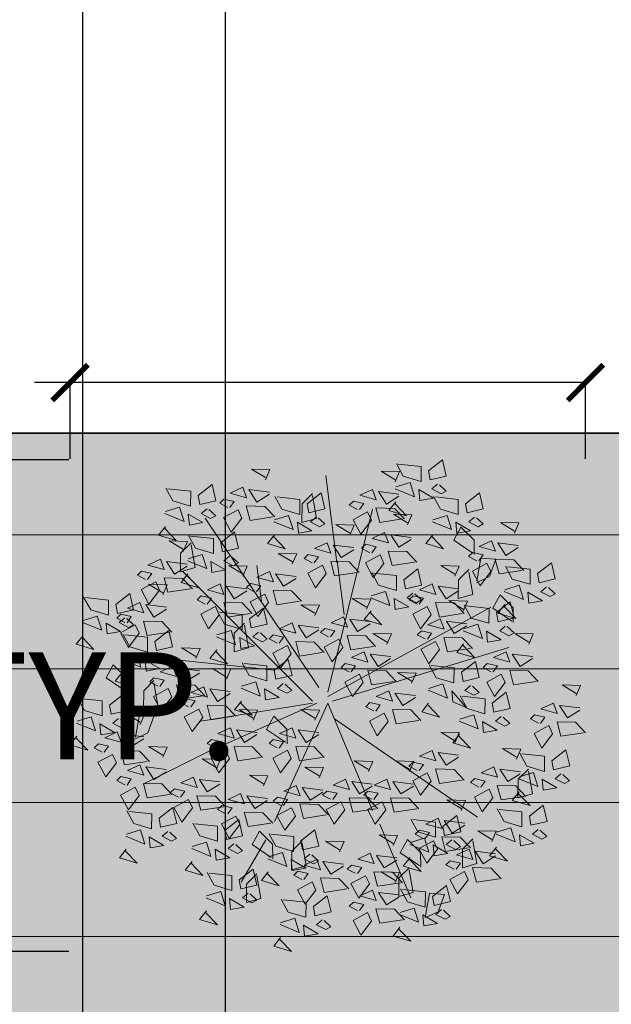
# Model space of a CAD drawing. Units: inches. Extents: x 1704 to 6393, y -157 to 1172.
# Tile 102 of 122: x 2594 to 2627, y 1001 to 1056. Entities that reach past the tile are written whole.
import ezdxf

# ---------------------------------------------------------------- set-up
doc = ezdxf.new("R2010")
doc.units = ezdxf.units.IN
doc.header["$MEASUREMENT"] = 0
for name, color, linetype, lineweight in [('A-ANNO-DIMS', 7, 'Continuous', 13), ('C-PROP', 7, 'Continuous', 35), ('L-DECK-PLNK-PATT', 250, 'Continuous', 13), ('L-shrub', 74, 'Continuous', 18)]:
    doc.layers.add(name, color=color, linetype=linetype, lineweight=lineweight)
doc.layers.add('L-DECK-PATT', color=35, linetype='Continuous', lineweight=13, true_color=0xa6725b)
doc.styles.get("Standard").update_dxf_attribs({"font": 'arial.ttf'})
doc.dimstyles.get("Standard").update_dxf_attribs({"dimtxt": 6, "dimasz": 2, "dimexe": 0.18, "dimexo": 0.0625, "dimgap": 0.09, "dimtad": 0, "dimtih": 1, "dimtoh": 1, "dimdec": 1, "dimzin": 0, "dimdsep": 46, "dimlunit": 3, "dimtxsty": 'Standard', "dimblk": 'ARCHTICK', "dimcen": 0.09, "dimadec": 0, "dimazin": 0, "dimtfac": 1, "dimtdec": 1, "dimtofl": 0, "dimtmove": 0, "dimatfit": 3, "dimfxl": 1, "dimtolj": 1, "dimtzin": 0, "dimarcsym": 0})

# ---------------------------------------------------------------- blocks, each defined once
blk = doc.blocks.new('flower shrub 3')
at = {"layer": 'L-shrub'}
for p, q in [((-123.5, 236), (-109, 242.8)), ((-109.8, 240.6), (-114, 215.7)), ((-130.4, 216.9), (-123.5, 236)), ((-114, 215.7), (-130.4, 216.9)), ((-96, 214.8), (-80.2, 219.2)), ((-80.2, 219.2), (-80.3, 198.9)), ((71.1, 221.6), (86.9, 226)), ((75.6, 196.7), (71.1, 221.6)), ((86.9, 226), (86.9, 205.7)), ((-91.6, 189.9), (-96, 214.8)), ((86.9, 205.7), (75.5, 194.4)), ((-80.3, 198.9), (-91.6, 187.7)), ((-166.1, 183.2), (-150.2, 187.7)), ((-150.2, 187.7), (-150.3, 167.3)), ((-104.3, 171), (-104.5, 187)), ((-102.9, 185.4), (-82, 171.2)), ((21.4, 185.5), (37.3, 189.9)), ((25.9, 160.6), (21.4, 185.5)), ((37.3, 189.9), (37.2, 169.6)), ((-161.6, 158.3), (-166.1, 183.2)), ((58.3, 162), (58.1, 177.9)), ((59.8, 176.3), (80.7, 162.2)), ((-150.3, 167.3), (-161.6, 156.1)), ((-89.8, 156.8), (-104.3, 171)), ((-82, 171.2), (-89.8, 156.8)), ((37.2, 169.6), (25.8, 158.3)), ((80.7, 162.2), (72.8, 147.7)), ((72.8, 147.7), (58.3, 162)), ((-227, 106.5), (-211.2, 110.9)), ((-211.2, 110.9), (-211.3, 90.6)), ((-222.6, 81.6), (-227, 106.5)), ((-211.3, 90.6), (-222.6, 79.4)), ((42.5, 35.6), (42.3, 51.6)), ((43.9, 50), (64.8, 35.8)), ((195.1, 39.7), (209.5, 46.5)), ((208.7, 44.3), (204.5, 19.5)), ((57, 21.4), (42.5, 35.6)), ((64.8, 35.8), (57, 21.4)), ((188.1, 20.6), (195.1, 39.7)), ((184.1, 9.5), (199.9, 13.9)), ((204.5, 19.5), (188.1, 20.6)), ((199.9, 13.9), (199.8, -6.4)), ((188.5, -15.4), (184.1, 9.5)), ((199.8, -6.4), (188.5, -17.7)), ((218.7, -20.8), (218.5, -4.8)), ((220.1, -6.4), (241, -20.6)), ((233.2, -35), (218.7, -20.8)), ((241, -20.6), (233.2, -35)), ((84.7, -53.7), (100.5, -49.2)), ((89.1, -78.6), (84.7, -53.7)), ((100.5, -49.2), (100.4, -69.6)), ((100.4, -69.6), (89.1, -80.8)), ((-206, -97.5), (-206.1, -81.5)), ((-204.5, -83.1), (-183.6, -97.3)), ((-191.5, -111.7), (-206, -97.5)), ((-183.6, -97.3), (-191.5, -111.7)), ((-161.5, -112.4), (-145.7, -107.9)), ((-145.7, -107.9), (-145.8, -128.2)), ((-157.1, -137.2), (-161.5, -112.4)), ((-179.9, -131.8), (-165.5, -125)), ((-166.2, -127.1), (-170.5, -152)), ((-145.8, -128.2), (-157.1, -139.5)), ((-186.9, -150.9), (-179.9, -131.8)), ((143.4, -141.7), (159.2, -137.2)), ((159.2, -137.2), (159.2, -157.6)), ((-170.5, -152), (-186.9, -150.9)), ((147.8, -166.6), (143.4, -141.7)), ((-163.1, -171.9), (-163.2, -156)), ((-161.6, -157.6), (-140.7, -171.7)), ((159.2, -157.6), (147.8, -168.8)), ((-148.6, -186.2), (-163.1, -171.9)), ((-140.7, -171.7), (-148.6, -186.2)), ((10.1, -195.8), (26, -191.4)), ((26, -191.4), (25.9, -211.7)), ((14.6, -220.7), (10.1, -195.8)), ((25.9, -211.7), (14.5, -223))]:
    blk.add_line(p, q, dxfattribs=at)
for points in [[(49.5, 264.4), (57, 273.9), (37.6, 279.7), (50.2, 266.6)], [(-81.5, 253.1), (-74, 262.7), (-93.5, 268.4), (-80.9, 255.3)], [(-50.4, 246.2), (-38.7, 261.6), (-30.1, 245.6), (-46.1, 237), (-50.4, 246.2)], [(24.3, 250.7), (23.1, 262.8), (8.2, 260.2), (24.3, 250.7)], [(-106.8, 239.4), (-107.9, 251.5), (-122.8, 248.9), (-106.8, 239.4)], [(-84.3, 244.8), (-59.4, 248.7), (-55.3, 232.7), (-75.6, 233.3), (-86.6, 244.9)], [(3.7, 245), (10, 250.2), (-0.2, 255.6), (-5.8, 252.5), (1.6, 245.7)], [(49.4, 248), (33.8, 243.2), (29, 258.7), (50, 250.1)], [(130.8, 235.1), (138.4, 244.6), (118.9, 250.4), (131.5, 237.2)], [(-127.3, 233.7), (-121, 238.9), (-131.2, 244.3), (-136.8, 241.3), (-129.5, 234.4)], [(-81.7, 236.7), (-97.2, 231.9), (-102, 247.4), (-81, 238.9)], [(13.5, 230.4), (-1.8, 218.4), (-6, 236.1), (11.8, 240.3), (13.5, 230.4)], [(46.7, 222.9), (21.5, 225.6), (21.7, 242.1), (41.2, 236.3), (48.8, 222.3)], [(-117.5, 219.1), (-132.8, 207.1), (-137, 224.8), (-119.3, 229), (-117.5, 219.1)], [(-84.4, 211.6), (-109.5, 214.3), (-109.3, 230.8), (-89.8, 225), (-82.2, 211)], [(-80.5, 219.9), (-66.7, 228.5), (-58, 214.8), (-80.5, 217.6)], [(-37.1, 234.5), (-41.8, 227.9), (-30.6, 225.3), (-26, 229.7), (-34.9, 234.5)], [(10.6, 212.3), (22.3, 227.8), (30.9, 211.8), (14.9, 203.2), (10.6, 212.3)], [(105.6, 221.4), (104.4, 233.5), (89.5, 230.8), (105.6, 221.4)], [(130.7, 218.7), (115.1, 213.8), (110.3, 229.4), (131.3, 220.8)], [(-156.6, 201), (-144.8, 216.5), (-136.2, 200.5), (-152.3, 191.9), (-156.6, 201)], [(-59.4, 140), (-93.7, 220.8)], [(-55.5, 223.7), (-51.3, 212.3), (-37.6, 218.7), (-55.5, 223.7)], [(-48.1, 205.5), (-36.4, 221), (-27.8, 205), (-43.9, 196.4), (-48.1, 205.5)], [(85, 215.7), (91.3, 220.9), (81.1, 226.3), (75.5, 223.2), (82.9, 216.3)], [(-82.1, 204.2), (-57.1, 208), (-53, 192.1), (-73.3, 192.7), (-84.3, 204.3)], [(-23.3, 211), (1.6, 214.8), (5.7, 198.9), (-14.6, 199.5), (-25.6, 211)], [(63.1, 192.2), (70.6, 201.7), (51.1, 207.5), (63.7, 194.4)], [(94.8, 201), (79.5, 189.1), (75.4, 206.8), (93.1, 211), (94.8, 201)], [(128, 193.6), (102.9, 196.3), (103, 212.7), (122.5, 207), (130.1, 192.9)], [(-190.5, 199.7), (-165.5, 203.5), (-161.4, 187.6), (-181.8, 188.2), (-192.7, 199.8)], [(-76.4, 204), (-81.2, 192.8), (-60.9, 192.3), (-76.4, 201.7)], [(-19.5, 186), (-5.7, 194.7), (3, 180.9), (-19.5, 183.8)], [(23.9, 200.7), (19.2, 194), (30.4, 191.5), (35, 195.9), (26.1, 200.6)], [(65.7, 157.2), (92.6, 203.7)], [(146.6, 180.9), (154.2, 190.5), (134.7, 196.2), (147.3, 183.1)], [(-143.3, 189.4), (-148, 182.7), (-136.8, 180.2), (-132.1, 184.6), (-141, 189.3)], [(-92.8, 176.4), (-85.3, 186), (-104.8, 191.7), (-92.2, 178.6)], [(-78.2, 179.3), (-64.4, 187.9), (-55.7, 174.2), (-78.3, 177)], [(-34.9, 193.9), (-39.6, 187.3), (-28.3, 184.7), (-23.7, 189.1), (-32.6, 193.8)], [(5.5, 189.9), (9.7, 178.5), (23.4, 184.9), (5.5, 189.9)], [(37.8, 178.5), (36.7, 190.6), (21.8, 188), (37.8, 178.5)], [(62.9, 175.8), (47.4, 171), (42.5, 186.5), (63.6, 177.9)], [(-187.7, 165.1), (-180.1, 174.7), (-199.6, 180.4), (-187, 167.3)], [(-186.6, 174.8), (-172.8, 183.4), (-164.2, 169.6), (-186.7, 172.5)], [(-161.7, 178.6), (-157.5, 167.2), (-143.7, 173.6), (-161.7, 178.6)], [(-118.1, 162.7), (-119.2, 174.8), (-134.1, 172.2), (-118.1, 162.7)], [(-122.7, 167.2), (-111, 182.7), (-102.3, 166.6), (-118.4, 158), (-122.7, 167.2)], [(-53.2, 183.1), (-49, 171.7), (-35.3, 178.1), (-53.2, 183.1)], [(17.3, 172.8), (23.5, 178), (13.3, 183.4), (7.7, 180.4), (15.1, 173.5)], [(121.4, 167.2), (120.3, 179.3), (105.3, 176.7), (121.4, 167.2)], [(146.5, 164.5), (130.9, 159.7), (126.1, 175.2), (147.1, 166.7)], [(218.9, 167.4), (226.5, 176.9), (207, 182.7), (219.6, 169.6)], [(-212.9, 151.4), (-214.1, 163.5), (-229, 160.9), (-212.9, 151.4)], [(-156.6, 165.8), (-131.6, 169.7), (-127.5, 153.8), (-147.9, 154.3), (-158.9, 165.9)], [(-138.6, 157), (-132.3, 162.2), (-142.5, 167.6), (-148.1, 164.6), (-140.8, 157.7)], [(-92.9, 160), (-108.5, 155.2), (-113.3, 170.7), (-92.3, 162.2)], [(-74.1, 163.4), (-78.9, 152.2), (-58.6, 151.7), (-74.2, 161.1)], [(-15.4, 170.1), (-20.2, 159), (0.1, 158.4), (-15.4, 167.9)], [(27.1, 158.2), (11.8, 146.2), (7.6, 163.9), (25.3, 168.1), (27.1, 158.2)], [(60.2, 150.7), (35.1, 153.4), (35.3, 169.9), (54.7, 164.1), (62.4, 150.1)], [(100.9, 161.5), (107.1, 166.7), (96.9, 172.1), (91.3, 169.1), (98.7, 162.2)], [(193.7, 153.7), (192.5, 165.8), (177.6, 163.1), (193.7, 153.7)], [(-233.5, 145.7), (-227.2, 151), (-237.4, 156.3), (-243, 153.3), (-235.6, 146.4)], [(-187.8, 148.7), (-203.4, 143.9), (-208.2, 159.4), (-187.2, 150.9)], [(-182.5, 158.9), (-187.4, 147.7), (-167, 147.1), (-182.6, 156.6)], [(-128.8, 142.4), (-144.1, 130.4), (-148.3, 148.1), (-130.6, 152.3), (-128.8, 142.4)], [(-95.7, 134.9), (-120.8, 137.6), (-120.6, 154.1), (-101.1, 148.3), (-93.5, 134.3)], [(-109.4, 155.5), (-114.1, 148.9), (-102.9, 146.3), (-98.3, 150.7), (-107.2, 155.5)], [(110.7, 146.9), (95.3, 134.9), (91.2, 152.6), (108.9, 156.8), (110.7, 146.9)], [(94.2, 140.1), (105.9, 155.6), (114.5, 139.6), (98.5, 131), (94.2, 140.1)], [(143.8, 139.4), (118.7, 142.1), (118.8, 158.6), (138.3, 152.8), (146, 138.8)], [(173.1, 148), (179.4, 153.2), (169.2, 158.6), (163.6, 155.5), (171, 148.6)], [(218.8, 151), (203.2, 146.2), (198.4, 161.7), (219.4, 153.1)], [(-223.7, 131.1), (-239, 119.1), (-243.2, 136.9), (-225.4, 141), (-223.7, 131.1)], [(-190.5, 123.6), (-215.6, 126.4), (-215.5, 142.8), (-196, 137), (-188.4, 123)], [(-152.8, 140.9), (-139, 149.6), (-130.3, 135.8), (-152.8, 138.7)], [(-127.8, 144.8), (-123.6, 133.4), (-109.9, 139.8), (-127.8, 144.8)], [(33.2, 131.1), (44.9, 146.6), (53.5, 130.5), (37.5, 121.9), (33.2, 131.1)], [(60.3, 138.8), (85.2, 142.6), (89.3, 126.7), (69, 127.3), (58, 138.8)], [(182.9, 133.3), (167.6, 121.4), (163.4, 139.1), (181.2, 143.3), (182.9, 133.3)], [(216.1, 125.9), (191, 128.6), (191.1, 145), (210.6, 139.3), (218.2, 125.2)], [(-9.9, 24.3), (-166.8, 132)], [(-66.2, 124.3), (-54.5, 139.8), (-45.9, 123.8), (-61.9, 115.2), (-66.2, 124.3)], [(-21, 124.3), (-9.3, 139.8), (-0.7, 123.8), (-16.7, 115.2), (-21, 124.3)], [(-0.7, 129.8), (24.2, 133.6), (28.3, 117.7), (8, 118.2), (-3, 129.8)], [(-2.5, 7.1), (56.3, 136.9)], [(146.1, 122.1), (157.9, 137.6), (166.5, 121.5), (150.4, 112.9), (146.1, 122.1)], [(-212.5, 104.2), (-205, 113.8), (-224.5, 119.5), (-211.9, 106.4)], [(-183.7, 110.8), (-171.9, 126.3), (-163.3, 110.2), (-179.4, 101.6), (-183.7, 110.8)], [(-148.7, 125), (-153.5, 113.9), (-133.2, 113.3), (-148.7, 122.8)], [(-100.1, 123), (-75.2, 126.8), (-71.1, 110.9), (-91.4, 111.5), (-102.4, 123)], [(-54.9, 123), (-30, 126.8), (-25.9, 110.9), (-46.2, 111.5), (-57.2, 123)], [(-2.5, 7.1), (-51.6, 124.7)], [(46.4, 119.4), (41.7, 112.8), (53, 110.2), (57.6, 114.6), (48.7, 119.4)], [(64.1, 113.8), (77.9, 122.5), (86.6, 108.7), (64, 111.6)], [(107.4, 128.5), (102.7, 121.8), (114, 119.3), (118.6, 123.7), (109.7, 128.4)], [(112.2, 120.7), (137.2, 124.6), (141.3, 108.7), (120.9, 109.2), (110, 120.8)], [(204.9, 108.5), (216.6, 124), (225.2, 108), (209.2, 99.4), (204.9, 108.5)], [(-217.6, 109.4), (-192.6, 113.3), (-188.5, 97.4), (-208.9, 97.9), (-219.9, 109.5)], [(-115.9, 92.7), (-104.2, 108.2), (-95.6, 92.2), (-111.6, 83.6), (-115.9, 92.7)], [(-53, 112.7), (-57.6, 106), (-46.4, 103.5), (-41.8, 107.9), (-50.7, 112.6)], [(-7.8, 112.7), (-12.5, 106), (-1.2, 103.5), (3.4, 107.9), (-5.5, 112.6)], [(3.1, 104.8), (16.9, 113.5), (25.6, 99.7), (3.1, 102.6)], [(28.1, 108.7), (32.3, 97.3), (46, 103.7), (28.1, 108.7)], [(89.1, 117.7), (93.3, 106.3), (107, 112.7), (89.1, 117.7)], [(159.4, 110.4), (154.7, 103.8), (165.9, 101.2), (170.6, 105.6), (161.6, 110.4)], [(170.9, 107.2), (195.9, 111), (200, 95.1), (179.7, 95.7), (168.7, 107.3)], [(-237.8, 90.5), (-238.9, 102.6), (-253.8, 100), (-237.8, 90.5)], [(-212.7, 87.8), (-228.2, 83), (-233.1, 98.5), (-212, 90)], [(-170.4, 99.1), (-175.1, 92.5), (-163.9, 89.9), (-159.2, 94.3), (-168.2, 99.1)], [(-96.3, 98.1), (-82.5, 106.7), (-73.8, 92.9), (-96.3, 95.8)], [(-71.3, 101.9), (-67.1, 90.5), (-53.4, 96.9), (-71.3, 101.9)], [(-51.1, 98.1), (-37.3, 106.7), (-28.6, 92.9), (-51.2, 95.8)], [(-26.1, 101.9), (-21.9, 90.5), (-8.2, 96.9), (-26.1, 101.9)], [(68.2, 97.9), (63.4, 86.8), (83.7, 86.2), (68.1, 95.7)], [(116.1, 95.8), (129.9, 104.5), (138.5, 90.7), (116, 93.5)], [(141, 99.6), (145.2, 88.2), (159, 94.6), (141, 99.6)], [(-258.3, 84.8), (-252.1, 90), (-262.2, 95.4), (-267.9, 92.4), (-260.5, 85.5)], [(-213.7, 84.5), (-200, 93.2), (-191.3, 79.4), (-213.8, 82.3)], [(-188.8, 88.4), (-184.6, 77), (-170.8, 83.4), (-188.8, 88.4)], [(-149.8, 91.4), (-124.9, 95.2), (-120.8, 79.3), (-141.1, 79.9), (-152.1, 91.5)], [(7.2, 88.9), (2.4, 77.8), (22.7, 77.2), (7.1, 86.7)], [(122.1, 56.8), (200.5, 95.9)], [(174.8, 82.3), (188.6, 90.9), (197.3, 77.1), (174.7, 80)], [(218.1, 96.9), (213.4, 90.2), (224.7, 87.7), (229.3, 92.1), (220.4, 96.8)], [(229.7, 72.4), (241.4, 87.9), (250.1, 71.9), (234, 63.3), (229.7, 72.4)], [(-248.5, 70.2), (-263.8, 58.2), (-268, 75.9), (-250.3, 80.1), (-248.5, 70.2)], [(-215.4, 62.7), (-240.5, 65.4), (-240.3, 81.9), (-220.8, 76.1), (-213.2, 62.1)], [(-102.6, 81.1), (-107.3, 74.5), (-96.1, 71.9), (-91.5, 76.3), (-100.4, 81)], [(-92.2, 82.1), (-97, 71), (-76.7, 70.4), (-92.3, 79.9)], [(-47, 82.1), (-51.8, 71), (-31.5, 70.4), (-47.1, 79.9)], [(37.7, 67.9), (49.4, 83.4), (58, 67.4), (42, 58.8), (37.7, 67.9)], [(105.5, 67.9), (117.2, 83.4), (125.8, 67.4), (109.8, 58.8), (105.5, 67.9)], [(120.2, 79.9), (115.3, 68.7), (135.7, 68.2), (120.1, 77.6)], [(199.8, 86.1), (204, 74.7), (217.7, 81.1), (199.8, 86.1)], [(-209.7, 68.6), (-214.5, 57.5), (-194.2, 56.9), (-209.7, 66.3)], [(-146, 66.5), (-132.2, 75.1), (-123.5, 61.3), (-146, 64.2)], [(-121, 70.3), (-116.8, 58.9), (-103.1, 65.3), (-121, 70.3)], [(3.8, 66.6), (28.7, 70.4), (32.8, 54.5), (12.5, 55.1), (1.5, 66.6)], [(71.6, 66.6), (96.5, 70.4), (100.6, 54.5), (80.3, 55.1), (69.3, 66.6)], [(178.9, 66.3), (174.1, 55.2), (194.4, 54.6), (178.8, 64.1)], [(195.8, 71.1), (220.8, 74.9), (224.8, 59), (204.5, 59.6), (193.5, 71.2)], [(-249.2, 40.8), (-237.5, 56.3), (-228.8, 40.3), (-244.9, 31.7), (-249.2, 40.8)], [(-147, 41), (-139.5, 50.6), (-159, 56.4), (-146.4, 43.2)], [(9.7, 7.1), (125, 58.6)], [(51, 56.3), (46.3, 49.6), (57.5, 47.1), (62.1, 51.5), (53.2, 56.2)], [(118.7, 56.3), (114, 49.6), (125.3, 47.1), (129.9, 51.5), (121, 56.2)], [(199.6, 46.2), (213.4, 54.8), (222.1, 41), (199.6, 43.9)], [(243, 60.8), (238.3, 54.1), (249.5, 51.6), (254.1, 56), (245.2, 60.7)], [(273.1, 43.3), (280.7, 52.8), (261.2, 58.6), (273.8, 45.5)], [(-283.1, 39.5), (-258.1, 43.3), (-254.1, 27.4), (-274.4, 28), (-285.4, 39.6)], [(-141.9, 50.6), (-146.7, 39.4), (-126.4, 38.9), (-141.9, 48.3)], [(7.6, 41.6), (21.4, 50.3), (30.1, 36.5), (7.6, 39.4)], [(32.6, 45.5), (36.8, 34.1), (50.5, 40.5), (32.6, 45.5)], [(75.4, 41.6), (89.2, 50.3), (97.9, 36.5), (75.3, 39.4)], [(100.4, 45.5), (104.6, 34.1), (118.3, 40.5), (100.4, 45.5)], [(224.6, 50), (228.8, 38.6), (242.5, 45), (224.6, 50)], [(-172.3, 27.3), (-173.4, 39.4), (-188.3, 36.8), (-172.3, 27.3)], [(-147.2, 24.6), (-162.7, 19.8), (-167.5, 35.4), (-146.5, 26.8)], [(-68.5, 27.3), (-56.7, 42.8), (-48.1, 26.8), (-64.2, 18.2), (-68.5, 27.3)], [(134.9, 22.8), (146.6, 38.3), (155.2, 22.2), (139.1, 13.7), (134.9, 22.8)], [(227.4, 23.9), (233.6, 29.1), (223.4, 34.5), (217.8, 31.4), (225.2, 24.6)], [(247.9, 29.6), (246.8, 41.7), (231.8, 39.1), (247.9, 29.6)], [(273, 26.9), (257.4, 22.1), (252.6, 37.6), (273.6, 29)], [(-279.3, 14.6), (-265.5, 23.2), (-256.8, 9.5), (-279.3, 12.3)], [(-235.9, 29.2), (-240.6, 22.6), (-229.4, 20), (-224.8, 24.4), (-233.7, 29.1)], [(-192.8, 21.7), (-186.5, 26.9), (-196.7, 32.2), (-202.4, 29.2), (-195, 22.3)], [(-113.1, 7.2), (-105.6, 16.7), (-125.1, 22.5), (-112.5, 9.4)], [(-102.4, 26), (-77.4, 29.8), (-73.3, 13.9), (-93.7, 14.4), (-104.6, 26)], [(11.7, 25.7), (6.9, 14.6), (27.2, 14), (11.7, 23.5)], [(14.6, 7.1), (137.2, 26.7)], [(79.5, 25.7), (74.7, 14.6), (95, 14), (79.4, 23.5)], [(100.9, 21.5), (125.9, 25.3), (130, 9.4), (109.6, 9.9), (98.7, 21.5)], [(203.7, 30.3), (198.9, 19.1), (219.2, 18.5), (203.7, 28)], [(-254.3, 18.4), (-250.1, 7), (-236.4, 13.4), (-254.3, 18.4)], [(-183, 7), (-198.3, -4.9), (-202.5, 12.8), (-184.8, 16.9), (-183, 7)], [(-149.9, -0.5), (-175, 2.3), (-174.8, 18.7), (-155.3, 12.9), (-147.7, -1.1)], [(-138.4, -6.5), (-139.5, 5.6), (-154.3, 11.9), (-138.4, -6.5)], [(-55.2, 15.7), (-59.9, 9), (-48.7, 6.5), (-44, 10.9), (-53, 15.6)], [(92.4, 4.9), (100, 14.5), (80.5, 20.3), (93.1, 7.1)], [(148.1, 11.2), (143.4, 4.5), (154.6, 2), (159.3, 6.3), (150.4, 11.1)], [(168.7, 0.2), (180.5, 15.7), (189.1, -0.3), (173, -8.9), (168.7, 0.2)], [(237.2, 9.2), (221.8, -2.7), (217.7, 15), (235.4, 19.2), (237.2, 9.2)], [(270.3, 1.8), (245.2, 4.5), (245.3, 20.9), (264.8, 15.2), (272.5, 1.2)], [(-7.4, 4.7), (-201.1, -54.1)], [(-113.3, -9.2), (-128.8, -14), (-133.7, 1.5), (-112.6, -7.1)], [(-98.5, 1), (-84.7, 9.7), (-76.1, -4.1), (-98.6, -1.2)], [(-73.6, 4.9), (-69.4, -6.5), (-55.6, -0.1), (-73.6, 4.9)], [(14.6, 4.7), (156.8, -137.4)], [(67.2, -8.8), (66, 3.3), (51.1, 0.7), (67.2, -8.8)], [(104.8, -3.5), (118.6, 5.2), (127.2, -8.6), (104.7, -5.7)], [(129.7, 0.4), (133.9, -11), (147.7, -4.6), (129.7, 0.4)], [(134.8, -1.1), (159.8, 2.7), (163.9, -13.2), (143.5, -12.6), (132.5, -1)], [(-275.2, -1.3), (-280, -12.5), (-259.7, -13), (-275.2, -3.6)], [(-197.2, -15.6), (-185.5, -0.1), (-176.9, -16.1), (-192.9, -24.7), (-197.2, -15.6)], [(-2.5, -0.2), (-181.5, -98.2)], [(-158.9, -12.2), (-152.7, -7), (-162.9, -1.6), (-168.5, -4.7), (-161.1, -11.5)], [(-2.5, -5.1), (-51.6, -205.9)], [(-41.3, -15.6), (-29.6, -0.1), (-21, -16.1), (-37.1, -24.7), (-41.3, -15.6)], [(7.3, -10), (132.3, -196.1)], [(46.6, -14.4), (52.9, -9.2), (42.7, -3.9), (37.1, -6.9), (44.5, -13.8)], [(92.3, -11.5), (76.7, -16.3), (71.9, -0.7), (92.9, -9.3)], [(-231.1, -16.9), (-206.2, -13.1), (-202.1, -29), (-222.4, -28.4), (-233.4, -16.8)], [(-149.1, -26.8), (-164.4, -38.8), (-168.6, -21.1), (-150.9, -16.9), (-149.1, -26.8)], [(-116, -34.3), (-141.1, -31.6), (-140.9, -15.2), (-121.5, -20.9), (-113.8, -34.9)], [(-94.4, -14.9), (-99.3, -26), (-78.9, -26.6), (-94.5, -17.1)], [(-75.3, -16.9), (-50.3, -13.1), (-46.2, -29), (-66.6, -28.4), (-77.5, -16.8)], [(56.4, -29.1), (41.1, -41), (36.9, -23.3), (54.7, -19.2), (56.4, -29.1)], [(89.6, -36.6), (64.5, -33.8), (64.6, -17.4), (84.1, -23.2), (91.7, -37.2)], [(108.9, -19.4), (104, -30.5), (124.4, -31.1), (108.8, -21.6)], [(138.6, -26), (152.4, -17.4), (161.1, -31.2), (138.6, -28.3)], [(182, -11.4), (177.3, -18.1), (188.5, -20.6), (193.1, -16.2), (184.2, -11.5)], [(223.5, -26.6), (231, -17.1), (211.5, -11.3), (224.1, -24.5)], [(-184, -27.2), (-188.7, -33.8), (-177.4, -36.4), (-172.8, -32), (-181.7, -27.3)], [(-28.1, -27.2), (-32.8, -33.8), (-21.6, -36.4), (-16.9, -32), (-25.8, -27.3)], [(37.7, -47.1), (49.4, -31.7), (58, -47.7), (42, -56.3), (37.7, -47.1)], [(55.9, -29), (171.1, -41.2)], [(163.6, -22.2), (167.8, -33.6), (181.6, -27.2), (163.6, -22.2)], [(198.2, -40.3), (197.1, -28.2), (182.1, -30.9), (198.2, -40.3)], [(223.3, -43.1), (207.7, -47.9), (202.9, -32.3), (223.9, -40.9)], [(-227.3, -41.8), (-213.5, -33.2), (-204.8, -46.9), (-227.4, -44.1)], [(-202.3, -38), (-198.1, -49.4), (-184.4, -43), (-202.3, -38)], [(-151.5, -58.2), (-144, -48.7), (-163.5, -42.9), (-150.9, -56.1)], [(-124.9, -51.7), (-113.2, -36.2), (-104.6, -52.2), (-120.7, -60.8), (-124.9, -51.7)], [(-71.4, -41.8), (-57.6, -33.2), (-49, -46.9), (-71.5, -44.1)], [(-46.5, -38), (-42.3, -49.4), (-28.5, -43), (-46.5, -38)], [(-18.8, -53.9), (-7, -38.4), (1.6, -54.5), (-14.5, -63.1), (-18.8, -53.9)], [(119.5, -51.5), (127.1, -41.9), (107.6, -36.2), (120.2, -49.3)], [(142.7, -41.9), (137.9, -53.1), (158.2, -53.6), (142.7, -44.2)], [(177.7, -46), (183.9, -40.8), (173.7, -35.5), (168.1, -38.5), (175.5, -45.4)], [(-158.9, -53), (-133.9, -49.2), (-129.8, -65.1), (-150.1, -64.5), (-161.1, -52.9)], [(-52.7, -55.3), (-27.7, -51.4), (-23.6, -67.3), (-44, -66.8), (-54.9, -55.2)], [(3.8, -48.5), (28.7, -44.6), (32.8, -60.6), (12.5, -60), (1.5, -48.4)], [(94.3, -65.2), (93.2, -53.1), (78.2, -55.7), (94.3, -65.2)], [(187.5, -60.7), (172.1, -72.6), (168, -54.9), (185.7, -50.8), (187.5, -60.7)], [(220.6, -68.1), (195.5, -65.4), (195.6, -49), (215.1, -54.8), (222.8, -68.8)], [(266.4, -67.2), (273.9, -57.7), (254.4, -51.9), (267, -65.1)], [(-223.2, -57.7), (-228, -68.9), (-207.7, -69.4), (-223.3, -60)], [(-176.8, -71.9), (-177.9, -59.8), (-192.8, -62.5), (-176.8, -71.9)], [(-151.7, -74.6), (-167.2, -79.5), (-172.1, -63.9), (-151, -72.5)], [(-111.7, -63.3), (-116.4, -69.9), (-105.2, -72.5), (-100.5, -68.1), (-109.4, -63.4)], [(-67.3, -57.7), (-72.2, -68.9), (-51.8, -69.4), (-67.4, -60)], [(7.6, -73.4), (21.4, -64.8), (30.1, -78.5), (7.6, -75.7)], [(51, -58.8), (46.3, -65.4), (57.5, -68), (62.1, -63.6), (53.2, -58.8)], [(73.8, -70.8), (80, -65.6), (69.8, -60.3), (64.2, -63.3), (71.6, -70.2)], [(119.4, -67.9), (103.8, -72.7), (99, -57.1), (120, -65.7)], [(204.9, -69.7), (216.6, -54.2), (225.2, -70.3), (209.2, -78.8), (204.9, -69.7)], [(-197.3, -77.6), (-191.1, -72.4), (-201.3, -67), (-206.9, -70.1), (-199.5, -77)], [(-155, -77.9), (-141.2, -69.3), (-132.6, -83), (-155.1, -80.2)], [(-130.1, -74.1), (-125.8, -85.5), (-112.1, -79.1), (-130.1, -74.1)], [(-115.9, -90), (-104.2, -74.5), (-95.6, -90.6), (-111.6, -99.2), (-115.9, -90)], [(-48.8, -80.2), (-35.1, -71.5), (-26.4, -85.3), (-48.9, -82.4)], [(-5.5, -65.6), (-10.2, -72.2), (1, -74.8), (5.7, -70.4), (-3.3, -65.6)], [(32.6, -69.6), (36.8, -81), (50.5, -74.6), (32.6, -69.6)], [(83.6, -85.5), (68.2, -97.4), (64.1, -79.7), (81.8, -75.6), (83.6, -85.5)], [(116.7, -93), (91.6, -90.2), (91.7, -73.8), (111.2, -79.6), (118.8, -93.6)], [(116.8, -90), (128.5, -74.5), (137.1, -90.6), (121.1, -99.2), (116.8, -90)], [(170.9, -71), (195.9, -67.2), (200, -83.1), (179.7, -82.6), (168.7, -71)], [(241.1, -80.9), (240, -68.9), (225.1, -71.5), (241.1, -80.9)], [(266.2, -83.7), (250.7, -88.5), (245.8, -72.9), (266.9, -81.5)], [(-196.7, -101.1), (-189.2, -91.6), (-208.7, -85.8), (-196.1, -98.9)], [(-187.5, -92.3), (-202.8, -104.2), (-207, -86.5), (-189.3, -82.3), (-187.5, -92.3)], [(-154.4, -99.7), (-179.5, -97), (-179.3, -80.6), (-159.9, -86.3), (-152.2, -100.4)], [(-49.9, -94.3), (-42.3, -84.8), (-61.8, -79), (-49.2, -92.2)], [(-23.9, -76.3), (-19.7, -87.7), (-5.9, -81.3), (-23.9, -76.3)], [(220.6, -86.6), (226.8, -81.4), (216.6, -76.1), (211, -79.1), (218.4, -86)], [(218.1, -81.3), (213.4, -88), (224.7, -90.6), (229.3, -86.2), (220.4, -81.4)], [(-150.9, -93.8), (-155.7, -105), (-135.4, -105.5), (-151, -96.1)], [(-149.8, -91.4), (-124.9, -87.5), (-120.8, -103.4), (-141.1, -102.9), (-152.1, -91.3)], [(-75.1, -108), (-76.3, -95.9), (-91.2, -98.6), (-75.1, -108)], [(-44.8, -96.1), (-49.6, -107.2), (-29.3, -107.8), (-44.8, -98.3)], [(-12.8, -149), (-20.2, -90.2)], [(11.7, -89.3), (6.9, -100.5), (27.2, -101), (11.7, -91.6)], [(62.6, -103.5), (74.3, -88.1), (82.9, -104.1), (66.8, -112.7), (62.6, -103.5)], [(82.8, -91.4), (107.8, -87.5), (111.9, -103.4), (91.6, -102.9), (80.6, -91.3)], [(174.8, -96), (188.6, -87.3), (197.3, -101.1), (174.7, -98.2)], [(199.8, -92.1), (204, -103.5), (217.7, -97.1), (199.8, -92.1)], [(230.4, -101.3), (215.1, -113.2), (210.9, -95.5), (228.6, -91.4), (230.4, -101.3)], [(263.5, -108.8), (238.4, -106), (238.6, -89.6), (258, -95.4), (265.7, -109.4)], [(-222, -114.8), (-223.1, -102.7), (-238, -105.3), (-222, -114.8)], [(-196.9, -117.5), (-212.4, -122.3), (-217.2, -106.8), (-196.2, -115.4)], [(-146, -116.3), (-132.2, -107.6), (-123.5, -121.4), (-146, -118.5)], [(-102.6, -101.7), (-107.3, -108.3), (-96.1, -110.9), (-91.5, -106.5), (-100.4, -101.7)], [(-95.7, -113.7), (-89.4, -108.5), (-99.6, -103.1), (-105.2, -106.2), (-97.8, -113.1)], [(-50, -110.7), (-65.6, -115.6), (-70.4, -100), (-49.4, -108.6)], [(28.6, -104.9), (53.6, -101), (57.7, -117), (37.4, -116.4), (26.4, -104.8)], [(70.6, -104.9), (75.5, -144.1)], [(86.7, -116.3), (100.5, -107.6), (109.2, -121.4), (86.6, -118.5)], [(130, -101.7), (125.3, -108.3), (136.6, -110.9), (141.2, -106.5), (132.3, -101.7)], [(182.3, -117.1), (194, -101.6), (202.6, -117.6), (186.6, -126.2), (182.3, -117.1)], [(-242.5, -120.5), (-236.2, -115.3), (-246.4, -109.9), (-252, -112.9), (-244.7, -119.8)], [(-121, -112.4), (-116.8, -123.8), (-103.1, -117.4), (-121, -112.4)], [(-85.9, -128.4), (-101.2, -140.3), (-105.4, -122.6), (-87.6, -118.4), (-85.9, -128.4)], [(-52.7, -135.8), (-77.8, -133.1), (-77.7, -116.7), (-58.2, -122.4), (-50.6, -136.5)], [(75.8, -115.2), (71.1, -121.8), (82.3, -124.4), (87, -120), (78.1, -115.3)], [(111.7, -112.4), (115.9, -123.8), (129.6, -117.4), (111.7, -112.4)], [(148.4, -118.4), (173.3, -114.6), (177.4, -130.5), (157.1, -129.9), (146.1, -118.4)], [(178.9, -111.9), (174.1, -123), (194.4, -123.6), (178.8, -114.1)], [(-232.7, -135.1), (-248, -147.1), (-252.2, -129.4), (-234.5, -125.2), (-232.7, -135.1)], [(-199.6, -142.6), (-224.7, -139.9), (-224.5, -123.4), (-205, -129.2), (-197.4, -143.2)], [(-181.4, -137.4), (-169.7, -121.9), (-161.1, -137.9), (-177.1, -146.5), (-181.4, -137.4)], [(-0.7, -135.1), (11, -119.7), (19.6, -135.7), (3.6, -144.3), (-0.7, -135.1)], [(32.5, -129.8), (46.3, -121.2), (54.9, -134.9), (32.4, -132.1)], [(57.4, -126), (61.7, -137.4), (75.4, -131), (57.4, -126)], [(151.2, -134.9), (158.7, -125.4), (139.2, -119.6), (151.8, -132.8)], [(195.5, -128.7), (190.8, -135.4), (202.1, -137.9), (206.7, -133.5), (197.8, -128.8)], [(-215.3, -138.7), (-190.4, -134.9), (-186.3, -150.8), (-206.6, -150.3), (-217.6, -138.7)], [(-141.9, -132.2), (-146.7, -143.3), (-126.4, -143.9), (-141.9, -134.4)], [(-63.9, -146.4), (-52.2, -130.9), (-43.6, -147), (-59.7, -155.6), (-63.9, -146.4)], [(-34.6, -136.5), (-9.7, -132.6), (-5.6, -148.5), (-25.9, -148), (-36.9, -136.4)], [(90.8, -132.2), (86, -143.3), (106.3, -143.9), (90.7, -134.4)], [(125.9, -148.6), (124.8, -136.5), (109.9, -139.2), (125.9, -148.6)], [(152.2, -143.4), (166, -134.7), (174.7, -148.5), (152.1, -145.6)], [(177.2, -139.5), (181.4, -150.9), (195.1, -144.5), (177.2, -139.5)], [(-168.2, -149), (-172.9, -155.7), (-161.6, -158.2), (-157, -153.8), (-165.9, -149.1)], [(-97.9, -147.8), (-72.9, -143.9), (-68.8, -159.8), (-89.1, -159.3), (-100.1, -147.7)], [(-12.3, -147.2), (-0.1, -242.7)], [(12.6, -146.8), (7.9, -153.4), (19.1, -156), (23.7, -151.6), (14.8, -146.8)], [(36.6, -145.7), (31.7, -156.9), (52.1, -157.4), (36.5, -148)], [(105.4, -154.3), (111.6, -149.1), (101.4, -143.7), (95.8, -146.8), (103.2, -153.7)], [(151, -151.4), (135.5, -156.2), (130.6, -140.6), (151.7, -149.2)], [(-211.5, -163.7), (-197.7, -155), (-189, -168.8), (-211.5, -165.9)], [(-186.5, -159.8), (-182.3, -171.2), (-168.6, -164.8), (-186.5, -159.8)], [(-50.7, -158.1), (-55.4, -164.7), (-44.2, -167.3), (-39.5, -162.9), (-48.4, -158.1)], [(-30.8, -161.4), (-17, -152.7), (-8.3, -166.5), (-30.8, -163.7)], [(-5.8, -157.6), (-1.6, -169), (12.1, -162.6), (-5.8, -157.6)], [(115.2, -169), (99.9, -180.9), (95.7, -163.2), (113.4, -159.1), (115.2, -169)], [(148.3, -176.4), (123.2, -173.7), (123.3, -157.3), (142.8, -163.1), (150.5, -177.1)], [(156.3, -159.3), (151.5, -170.4), (171.8, -171), (156.2, -161.5)], [(-117.6, -177.8), (-110.1, -168.3), (-129.6, -162.5), (-117, -175.6)], [(-94, -172.7), (-80.2, -164), (-71.6, -177.8), (-94.1, -174.9)], [(-69.1, -168.8), (-64.8, -180.2), (-51.1, -173.8), (-69.1, -168.8)], [(56.3, -177.8), (63.8, -168.3), (44.3, -162.5), (56.9, -175.6)], [(176, -186.8), (183.5, -177.3), (164.1, -171.5), (176.7, -184.7)], [(-207.4, -179.6), (-212.2, -190.7), (-191.9, -191.3), (-207.5, -181.8)], [(-142.9, -191.5), (-144, -179.4), (-159, -182), (-142.9, -191.5)], [(-117.8, -194.2), (-133.4, -199), (-138.2, -183.5), (-117.2, -192.1)], [(-50.4, -193.8), (-38.7, -178.3), (-30.1, -194.3), (-46.1, -202.9), (-50.4, -193.8)], [(-26.7, -177.3), (-31.5, -188.5), (-11.2, -189), (-26.7, -179.6)], [(31, -191.5), (29.9, -179.4), (15, -182), (31, -191.5)], [(56.1, -194.2), (40.6, -199), (35.8, -183.5), (56.8, -192.1)], [(91.9, -196.1), (103.6, -180.6), (112.3, -196.6), (96.2, -205.2), (91.9, -196.1)], [(-163.4, -197.2), (-157.2, -192), (-167.4, -186.6), (-173, -189.7), (-165.6, -196.5)], [(-89.9, -188.6), (-94.8, -199.8), (-74.4, -200.3), (-90, -190.9)], [(-84.3, -195.1), (-59.4, -191.3), (-55.3, -207.2), (-75.6, -206.7), (-86.6, -195.1)], [(10.5, -197.2), (16.8, -192), (6.6, -186.6), (1, -189.7), (8.3, -196.5)], [(58, -197.4), (83, -193.6), (87.1, -209.5), (66.7, -208.9), (55.7, -197.3)], [(150.8, -200.5), (149.6, -188.4), (134.7, -191.1), (150.8, -200.5)], [(175.9, -203.3), (160.3, -208.1), (155.5, -192.5), (176.5, -201.1)], [(-153.6, -211.9), (-169, -223.8), (-173.1, -206.1), (-155.4, -201.9), (-153.6, -211.9)], [(-120.5, -219.3), (-145.6, -216.6), (-145.5, -200.2), (-126, -205.9), (-118.3, -219.9)], [(-77, -213.9), (-69.5, -204.4), (-88.9, -198.6), (-76.3, -211.7)], [(20.3, -211.9), (5, -223.8), (0.8, -206.1), (18.5, -201.9), (20.3, -211.9)], [(53.4, -219.3), (28.3, -216.6), (28.5, -200.2), (48, -205.9), (55.6, -219.9)], [(130.2, -206.2), (136.5, -201), (126.3, -195.6), (120.7, -198.7), (128.1, -205.6)], [(-102.2, -227.6), (-103.4, -215.5), (-118.3, -218.1), (-102.2, -227.6)], [(-80.5, -220.1), (-66.7, -211.4), (-58, -225.2), (-80.5, -222.3)], [(-37.1, -205.4), (-41.8, -212.1), (-30.6, -214.6), (-26, -210.3), (-34.9, -205.5)], [(61.8, -222.3), (75.6, -213.7), (84.3, -227.4), (61.8, -224.6)], [(105.2, -207.7), (100.5, -214.3), (111.7, -216.9), (116.3, -212.5), (107.4, -207.8)], [(140, -220.9), (124.7, -232.8), (120.5, -215.1), (138.3, -210.9), (140, -220.9)], [(173.2, -228.3), (148, -225.6), (148.2, -209.2), (167.7, -214.9), (175.3, -229)], [(-122.8, -233.3), (-116.5, -228.1), (-126.7, -222.7), (-132.3, -225.8), (-124.9, -232.6)], [(-77.1, -230.3), (-92.7, -235.1), (-97.5, -219.6), (-76.5, -228.2)], [(-55.5, -216.2), (-51.3, -227.6), (-37.6, -221.2), (-55.5, -216.2)], [(86.8, -218.5), (91, -229.9), (104.7, -223.5), (86.8, -218.5)], [(-79.8, -255.4), (-105, -252.7), (-104.8, -236.3), (-85.3, -242), (-77.7, -256)], [(-76.4, -236), (-81.2, -247.1), (-60.9, -247.7), (-76.4, -238.2)], [(-113, -248), (-128.3, -259.9), (-132.5, -242.2), (-114.7, -238), (-113, -248)], [(65.9, -238.2), (61.1, -249.4), (81.4, -249.9), (65.9, -240.5)]]:
    blk.add_lwpolyline(points, dxfattribs=at)
blk = doc.blocks.new('_ArchTick')
at = {"color": 0, "linetype": 'ByBlock', "const_width": 0.15}
blk.add_lwpolyline([(-0.5, -0.5), (0.5, 0.5)], dxfattribs=at)
blk = doc.blocks.new('*D88')
at = {"layer": 'A-ANNO-DIMS', "color": 0, "lineweight": -2, "transparency": 16777216}
for p, q in [((2596.639, 1036.042), (2594.639, 1036.042)), ((2596.639, 1031.77), (2596.639, 1036.222)), ((2625.54, 1036.042), (2596.639, 1036.042)), ((2625.54, 1031.77), (2625.54, 1036.222))]:
    blk.add_line(p, q, dxfattribs=at)
at = {"layer": 'Defpoints', "color": 0, "lineweight": -3, "transparency": 16777216}
for p in [(2596.639, 1036.042), (2596.639, 1031.707), (2625.54, 1031.707)]:
    blk.add_point(p, dxfattribs=at)
at = {"layer": 'A-ANNO-DIMS', "color": 0, "lineweight": -2, "transparency": 16777216, "xscale": 2, "yscale": 2, "zscale": 2, "rotation": 180}
blk.add_blockref('_ArchTick', (2596.639, 1036.042), dxfattribs=at)
at = {"layer": 'A-ANNO-DIMS', "color": 0, "lineweight": -2, "transparency": 16777216, "xscale": 2, "yscale": 2, "zscale": 2}
blk.add_blockref('_ArchTick', (2625.54, 1036.042), dxfattribs=at)
at = {"layer": 'A-ANNO-DIMS', "color": 0, "transparency": 16777216, "insert": (2560.165, 1036.042), "char_height": 6, "attachment_point": 5}
blk.add_mtext('\\A1;SHRUB A 29 TYP.', dxfattribs=at)
blk = doc.blocks.new('*D89')
at = {"layer": 'A-ANNO-DIMS', "color": 0, "lineweight": -2, "transparency": 16777216}
for p, q in [((2596.576, 1031.707), (2592.123, 1031.707)), ((2592.303, 1031.707), (2592.303, 1021.085)), ((2592.303, 1004.156), (2592.303, 1014.778)), ((2596.576, 1004.156), (2592.123, 1004.156))]:
    blk.add_line(p, q, dxfattribs=at)
at = {"layer": 'Defpoints', "color": 0, "lineweight": -3, "transparency": 16777216}
for p in [(2596.639, 1031.707), (2592.303, 1004.156), (2596.639, 1004.156)]:
    blk.add_point(p, dxfattribs=at)
at = {"layer": 'A-ANNO-DIMS', "color": 0, "lineweight": -2, "transparency": 16777216, "xscale": 2, "yscale": 2, "zscale": 2}
for p, rotation in [((2592.303, 1031.707), 90), ((2592.303, 1004.156), 270)]:
    blk.add_blockref('_ArchTick', p, dxfattribs=dict(at, rotation=rotation))
at = {"layer": 'A-ANNO-DIMS', "color": 0, "transparency": 16777216, "insert": (2592.303, 1017.931), "char_height": 6, "attachment_point": 5}
blk.add_mtext('\\A1;28 TYP.', dxfattribs=at)
blk = doc.blocks.new('*D92')
at = {"layer": 'A-ANNO-DIMS', "color": 0, "lineweight": -2, "transparency": 16777216}
for p, q in [((2073.349, 895.275), (2073.349, 1105.287)), ((2605.349, 895.275), (2605.349, 1105.287)), ((2073.349, 1105.107), (2332.661, 1105.107)), ((2605.349, 1105.107), (2346.036, 1105.107))]:
    blk.add_line(p, q, dxfattribs=at)
at = {"layer": 'Defpoints', "color": 0, "lineweight": -3, "transparency": 16777216}
for p in [(2605.349, 1105.107), (2073.349, 895.213), (2605.349, 895.213)]:
    blk.add_point(p, dxfattribs=at)
at = {"layer": 'A-ANNO-DIMS', "color": 0, "lineweight": -2, "transparency": 16777216, "xscale": 2, "yscale": 2, "zscale": 2, "rotation": 180}
blk.add_blockref('_ArchTick', (2073.349, 1105.107), dxfattribs=at)
at = {"layer": 'A-ANNO-DIMS', "color": 0, "lineweight": -2, "transparency": 16777216, "xscale": 2, "yscale": 2, "zscale": 2}
blk.add_blockref('_ArchTick', (2605.349, 1105.107), dxfattribs=at)
at = {"layer": 'A-ANNO-DIMS', "color": 0, "transparency": 16777216, "insert": (2339.349, 1105.107), "char_height": 6, "attachment_point": 5}
blk.add_mtext('\\A1;532', dxfattribs=at)
blk = doc.blocks.new('*D95')
at = {"layer": 'A-ANNO-DIMS', "color": 0, "lineweight": -2, "transparency": 16777216}
for p, q in [((2605.349, 895.275), (2605.349, 1105.287)), ((2723.349, 895.275), (2723.349, 1105.287)), ((2605.349, 1105.107), (2657.907, 1105.107)), ((2723.349, 1105.107), (2670.791, 1105.107))]:
    blk.add_line(p, q, dxfattribs=at)
at = {"layer": 'Defpoints', "color": 0, "lineweight": -3, "transparency": 16777216}
for p in [(2723.349, 1105.107), (2605.349, 895.213), (2723.349, 895.213)]:
    blk.add_point(p, dxfattribs=at)
at = {"layer": 'A-ANNO-DIMS', "color": 0, "lineweight": -2, "transparency": 16777216, "xscale": 2, "yscale": 2, "zscale": 2, "rotation": 180}
blk.add_blockref('_ArchTick', (2605.349, 1105.107), dxfattribs=at)
at = {"layer": 'A-ANNO-DIMS', "color": 0, "lineweight": -2, "transparency": 16777216, "xscale": 2, "yscale": 2, "zscale": 2}
blk.add_blockref('_ArchTick', (2723.349, 1105.107), dxfattribs=at)
at = {"layer": 'A-ANNO-DIMS', "color": 0, "transparency": 16777216, "insert": (2664.349, 1105.107), "char_height": 6, "attachment_point": 5}
blk.add_mtext('\\A1;118', dxfattribs=at)
blk = doc.blocks.new('*D103')
at = {"layer": 'A-ANNO-DIMS', "color": 0, "lineweight": -2, "transparency": 16777216}
for p, q in [((2551.349, 711.275), (2551.349, 1105.287)), ((2597.349, 711.275), (2597.349, 1105.287)), ((2551.349, 1105.107), (2569.842, 1105.107)), ((2597.349, 1105.107), (2578.855, 1105.107))]:
    blk.add_line(p, q, dxfattribs=at)
at = {"layer": 'Defpoints', "color": 0, "lineweight": -3, "transparency": 16777216}
for p in [(2597.349, 1105.107), (2551.349, 711.213), (2597.349, 711.213)]:
    blk.add_point(p, dxfattribs=at)
at = {"layer": 'A-ANNO-DIMS', "color": 0, "lineweight": -2, "transparency": 16777216, "xscale": 2, "yscale": 2, "zscale": 2, "rotation": 180}
blk.add_blockref('_ArchTick', (2551.349, 1105.107), dxfattribs=at)
at = {"layer": 'A-ANNO-DIMS', "color": 0, "lineweight": -2, "transparency": 16777216, "xscale": 2, "yscale": 2, "zscale": 2}
blk.add_blockref('_ArchTick', (2597.349, 1105.107), dxfattribs=at)
at = {"layer": 'A-ANNO-DIMS', "color": 0, "transparency": 16777216, "insert": (2574.349, 1105.107), "char_height": 6, "attachment_point": 5}
blk.add_mtext('\\A1;46', dxfattribs=at)

msp = doc.modelspace()

# ---------------------------------------------------------------- hatches: boundary and pattern name
at = {"layer": 'L-DECK-PATT', "transparency": 33554544}
h = msp.add_hatch(color=256, dxfattribs=at)
h.dxf.hatch_style = 1
h.paths.add_polyline_path([(2329.589, 1033.213), (2065.589, 1033.213), (2065.589, 895.213), (2167.349, 895.213), (2263.349, 895.213), (2263.349, 903.213), (2273.349, 903.213), (2273.349, 895.213), (2329.589, 895.213)])
h.paths.add_polyline_path([(2664.349, 1033.213), (2333.589, 1033.213), (2333.589, 895.213), (2465.349, 895.213), (2469.181, 895.213), (2470.482, 895.213), (2508.215, 895.213), (2509.516, 895.213), (2513.349, 895.213), (2533.349, 895.213), (2581.349, 895.213), (2605.349, 895.213), (2664.349, 895.213)])
h.paths.add_polyline_path([(2333.589, 1033.213), (2329.589, 1033.213), (2329.589, 895.213), (2333.589, 895.213)])
at = {"layer": 'L-DECK-PLNK-PATT'}
h = msp.add_hatch(dxfattribs=at)
h.set_pattern_fill('LINE', color=256, scale=60)
h.paths.add_polyline_path([(2329.589, 1033.213), (2065.589, 1033.213), (2065.589, 895.213), (2167.349, 895.213), (2263.349, 895.213), (2263.349, 903.213), (2273.349, 903.213), (2273.349, 895.213), (2329.589, 895.213)])
h.paths.add_polyline_path([(2664.349, 1033.213), (2333.589, 1033.213), (2333.589, 895.213), (2465.349, 895.213), (2469.181, 895.213), (2470.482, 895.213), (2508.215, 895.213), (2509.516, 895.213), (2513.349, 895.213), (2533.349, 895.213), (2581.349, 895.213), (2605.349, 895.213), (2664.349, 895.213)])
h.paths.add_polyline_path([(2333.589, 1033.213), (2329.589, 1033.213), (2329.589, 895.213), (2333.589, 895.213)])

# ---------------------------------------------------------------- linework, layer by layer
at = {"layer": 'C-PROP'}
msp.add_line((2723.349, 1033.213), (1898.349, 1033.213), dxfattribs=at)

# ---------------------------------------------------------------- block references
at = {"layer": 'L-shrub', "xscale": 0.0510581485411622, "yscale": 0.0510581485411622, "zscale": 0.0510581485411622, "rotation": 180}
msp.add_blockref('flower shrub 3', (2610.97, 1018.437), dxfattribs=at)

# ---------------------------------------------------------------- dimensions: what is measured, and where the dimension line sits
at = {"layer": 'A-ANNO-DIMS'}
for base, p1, p2, picture, middle in [((2605.349, 1105.107), (2073.349, 895.213), (2605.349, 895.213), '*D92', (2339.349, 1105.107)), ((2597.349, 1105.107), (2551.349, 711.213), (2597.349, 711.213), '*D103', (2574.349, 1105.107)), ((2723.349, 1105.107), (2605.349, 895.213), (2723.349, 895.213), '*D95', (2664.349, 1105.107))]:
    dim = msp.add_linear_dim(base=base, p1=p1, p2=p2, dimstyle='Standard', override={"dimdec": 0, "dimlfac": 1, "dimrnd": 0, "dimzin": 0, "dimdsep": 46, "dimlunit": 2}, dxfattribs=at)
    dim.commit()
    dim.dimension.update_dxf_attribs({"geometry": picture, "text_midpoint": middle})
for base, p1, p2, angle, text, picture, middle in [((2596.639, 1036.042), (2625.54, 1031.707), (2596.639, 1031.707), 180, 'SHRUB A <> TYP.', '*D88', (2560.165, 1036.042)), ((2592.303, 1004.156), (2596.639, 1031.707), (2596.639, 1004.156), 270, '<> TYP.', '*D89', (2592.303, 1017.931))]:
    dim = msp.add_linear_dim(base=base, p1=p1, p2=p2, angle=angle, text=text, dimstyle='Standard', override={"dimdec": 0, "dimlfac": 1, "dimrnd": 0, "dimzin": 0, "dimdsep": 46, "dimlunit": 2}, dxfattribs=at)
    dim.commit()
    dim.dimension.update_dxf_attribs({"geometry": picture, "text_midpoint": middle})

doc.saveas('drawing.dxf')
